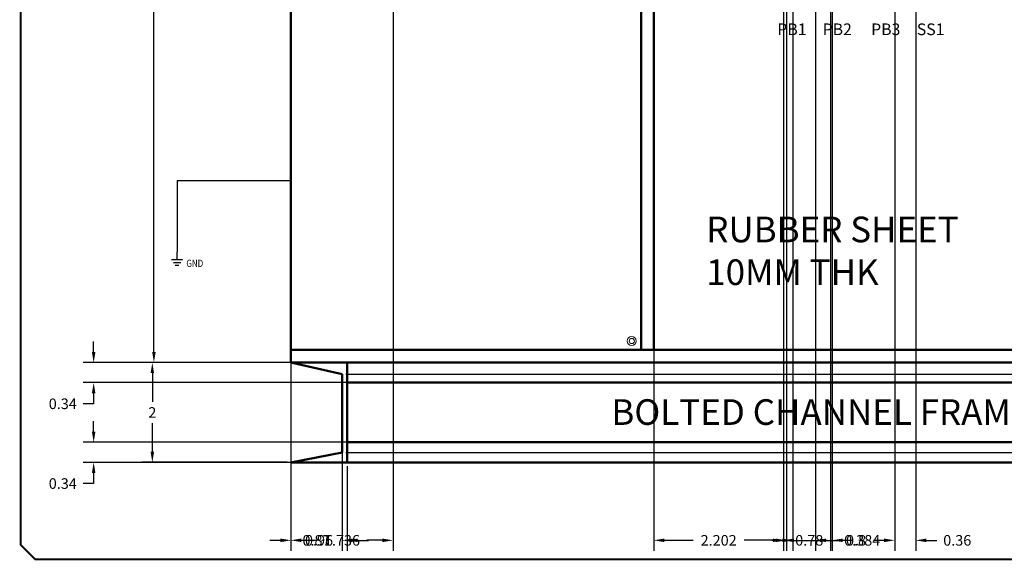
# Model space of a CAD drawing. Units: inches. Extents: x 0 to 33.5, y 0 to 22.4.
# Tile 1 of 6: x 0 to 16.8, y 0 to 9.2. Entities that reach past the tile are written whole.
import ezdxf
from ezdxf.enums import TextEntityAlignment as Align

# ---------------------------------------------------------------- set-up
doc = ezdxf.new("R2010")
doc.units = ezdxf.units.IN
doc.header["$MEASUREMENT"] = 0
for name, color, linetype, lineweight in [('E-ANNO-DIMS', 2, 'Continuous', 18), ('E-ANNO-TEXT', 7, 'Continuous', 18), ('E-ANNO-TTLB', 7, 'Continuous', 35), ('E-GRND-WIRE', 3, 'Continuous', 25), ('E-PANL-HDWR', 8, 'Continuous', 18), ('E-PANL-OUTL', 7, 'Continuous', 50), ('SYMS', 7, 'Continuous', 25)]:
    doc.layers.add(name, color=color, linetype=linetype, lineweight=lineweight)
doc.layers.add('TAGS', color=150, linetype='Continuous')
doc.layers.add('TITLE', color=7, linetype='Continuous')
doc.styles.add('ITALIC', font='ITALIC')
doc.styles.add('SIMPLEX', font='SIMPLEX')
doc.styles.add('WD', font='romans.shx')
doc.dimstyles.get("Standard").update_dxf_attribs({"dimtxt": 0.18, "dimasz": 0.18, "dimexe": 0.18, "dimexo": 0.0625, "dimgap": 0.09, "dimtad": 0, "dimtih": 1, "dimtoh": 1, "dimdec": 0, "dimzin": 0, "dimdsep": 46, "dimtxsty": 'Standard', "dimcen": 0.09, "dimadec": 0, "dimazin": 0, "dimtfac": 1, "dimtdec": 0, "dimtofl": 0, "dimtmove": 0, "dimatfit": 3, "dimfxl": 1, "dimtolj": 1, "dimtzin": 0, "dimarcsym": 0})

# ---------------------------------------------------------------- blocks, each defined once
blk = doc.blocks.new('NO_NUM_acade_title')
at = {"layer": 'TITLE', "const_width": 0.0312}
blk.add_lwpolyline([(30.594, 0.281), (30.594, 22.177), (30.344, 22.427), (0.281, 22.427), (0.031, 22.177), (0.031, 0.281), (0.281, 0.031), (30.344, 0.031)], close=True, dxfattribs=at)
at = {"layer": 'TITLE', "style": 'ITALIC'}
for tag, height, p in [('TITLE#1', 0.125, (32.156, 3.406)), ('TITLE#2', 0.125, (32.156, 3.204)), ('TITLE#3', 0.125, (32.156, 3.001)), ('TITLE#4', 0.125, (32.156, 2.799)), ('DWG#', 0.2, (32.156, 0.826))]:
    blk.add_attdef(tag, text='', height=height, dxfattribs=at).set_placement(p, align=Align.CENTER)
at = {"layer": 'TITLE', "style": 'SIMPLEX'}
blk.add_attdef('CAD#', (30.826, 1.958), '', height=0.0938, rotation=90, dxfattribs=at)
at = {"layer": 'TITLE'}
for tag, p, height, style in [('JOB#', (31.464, 1.644), 0.0938, 'SIMPLEX'), ('SCALE', (31.353, 1.344), 0.0938, 'SIMPLEX'), ('DATE', (32.408, 1.344), 0.0938, 'SIMPLEX'), ('SHTS', (32.532, 0.25), 0.2, 'ITALIC')]:
    blk.add_attdef(tag, p, '', height=height, dxfattribs=dict(at, style=style))
at = {"layer": 'TITLE', "style": 'ITALIC'}
blk.add_attdef('SH#', text='', height=0.2, dxfattribs=at).set_placement((31.881, 0.25), align=Align.RIGHT)
at = {"layer": 'TITLE', "flags": 9}
blk.add_attdef('WD_TB', (31.219, 0.031), '', height=0.125, dxfattribs=at)
blk = doc.blocks.new('VGND2')
for p, q in [((0, -0.125), (0, 0)), ((0.09375, -0.125), (-0.09375, -0.125)), ((-0.0625, -0.171875), (0.0625, -0.171875)), ((-0.03125, -0.21875), (0.03125, -0.21875))]:
    blk.add_line(p, q)
at = {"style": 'WD', "width": 0.8}
for tag, p in [('INST', (0.15625, 0.125)), ('LOC', (0.15625, -0.03125)), ('TAG1', (0.15625, -0.1875)), ('DESC1', (0.15625, -0.34375)), ('DESC2', (0.15625, -0.5))]:
    blk.add_attdef(tag, text='', height=0.125, dxfattribs=at).set_placement(p, align=Align.MIDDLE_LEFT)
at = {"style": 'WD', "flags": 1}
for tag in ['ASSYCODE', 'X2TERM01', 'CAT', 'MFG', 'FAMILY']:
    blk.add_attdef(tag, (0, 0), '', height=0.01, dxfattribs=at)
blk = doc.blocks.new('*D17')
at = {"layer": 'Defpoints', "color": 0, "transparency": 16777216}
for p in [(4.625, 18.375), (2.297, 3.375), (4.625, 3.375)]:
    blk.add_point(p, dxfattribs=at)
at = {"layer": 'E-ANNO-DIMS', "color": 0, "lineweight": -2, "transparency": 16777216}
for p, q in [((4.563, 18.375), (2.117, 18.375)), ((2.297, 18.195), (2.297, 11.055)), ((2.297, 3.555), (2.297, 10.695)), ((4.563, 3.375), (2.117, 3.375))]:
    blk.add_line(p, q, dxfattribs=at)
at = {"layer": 'E-ANNO-DIMS', "color": 0, "transparency": 16777216}
for points in [[(2.267, 18.195), (2.327, 18.195), (2.297, 18.375)], [(2.267, 3.555), (2.327, 3.555), (2.297, 3.375)]]:
    blk.add_solid(points, dxfattribs=at)
at = {"layer": 'E-ANNO-DIMS', "color": 0, "transparency": 16777216, "insert": (2.297, 10.875), "char_height": 0.18, "attachment_point": 5}
blk.add_mtext('\\A1;15', dxfattribs=at)
blk = doc.blocks.new('*D21')
at = {"layer": 'Defpoints', "color": 0, "transparency": 16777216}
for p in [(2.27, 3.375), (4.625, 3.375), (4.625, 1.68)]:
    blk.add_point(p, dxfattribs=at)
at = {"layer": 'E-ANNO-DIMS', "color": 0, "lineweight": -2, "transparency": 16777216}
for p, q in [((4.563, 3.375), (2.09, 3.375)), ((2.27, 3.195), (2.27, 2.707)), ((2.27, 1.86), (2.27, 2.347)), ((4.563, 1.68), (2.09, 1.68))]:
    blk.add_line(p, q, dxfattribs=at)
at = {"layer": 'E-ANNO-DIMS', "color": 0, "transparency": 16777216}
for points in [[(2.24, 3.195), (2.3, 3.195), (2.27, 3.375)], [(2.24, 1.86), (2.3, 1.86), (2.27, 1.68)]]:
    blk.add_solid(points, dxfattribs=at)
at = {"layer": 'E-ANNO-DIMS', "color": 0, "transparency": 16777216, "insert": (2.27, 2.527), "char_height": 0.18, "attachment_point": 5}
blk.add_mtext('\\A1;2', dxfattribs=at)
blk = doc.blocks.new('SCREW-PANEL')
for radius in [0.0768, 0.0442]:
    blk.add_circle((0.077, 0.077), radius)
blk = doc.blocks.new('*D27')
at = {"layer": 'Defpoints', "color": 0, "transparency": 16777216}
for p in [(13.540199, 20.522539), (13.156258, 18.375), (13.540199, 0.354641)]:
    blk.add_point(p, dxfattribs=at)
at = {"layer": 'E-ANNO-DIMS', "color": 0, "lineweight": -2, "transparency": 16777216}
for p, q in [((13.540199, 20.460039), (13.540199, 0.174641)), ((13.156258, 18.3125), (13.156258, 0.174641)), ((12.976258, 0.354641), (12.796258, 0.354641)), ((13.720199, 0.354641), (13.900199, 0.354641))]:
    blk.add_line(p, q, dxfattribs=at)
at = {"layer": 'E-ANNO-DIMS', "color": 0, "transparency": 16777216}
for points in [[(12.976258, 0.384641), (12.976258, 0.324641), (13.156258, 0.354641)], [(13.720199, 0.384641), (13.720199, 0.324641), (13.540199, 0.354641)]]:
    blk.add_solid(points, dxfattribs=at)
at = {"layer": 'E-ANNO-DIMS', "color": 0, "transparency": 16777216, "insert": (14.335199, 0.354641), "char_height": 0.18, "attachment_point": 5}
blk.add_mtext('\\A1;0.384', dxfattribs=at)
blk = doc.blocks.new('*D28')
at = {"layer": 'Defpoints', "color": 0, "transparency": 16777216}
for p in [(14.887335, 20.522539), (15.245612, 18.375), (15.245612, 0.354641)]:
    blk.add_point(p, dxfattribs=at)
at = {"layer": 'E-ANNO-DIMS', "color": 0, "lineweight": -2, "transparency": 16777216}
for p, q in [((14.887335, 20.460039), (14.887335, 0.174641)), ((15.245612, 18.3125), (15.245612, 0.174641)), ((14.707335, 0.354641), (14.527335, 0.354641)), ((15.425612, 0.354641), (15.605612, 0.354641))]:
    blk.add_line(p, q, dxfattribs=at)
at = {"layer": 'E-ANNO-DIMS', "color": 0, "transparency": 16777216}
for points in [[(14.707335, 0.384641), (14.707335, 0.324641), (14.887335, 0.354641)], [(15.425612, 0.384641), (15.425612, 0.324641), (15.245612, 0.354641)]]:
    blk.add_solid(points, dxfattribs=at)
at = {"layer": 'E-ANNO-DIMS', "color": 0, "transparency": 16777216, "insert": (15.950612, 0.354641), "char_height": 0.18, "attachment_point": 5}
blk.add_mtext('\\A1;0.36', dxfattribs=at)
blk = doc.blocks.new('*D31')
at = {"layer": 'Defpoints', "color": 0, "transparency": 16777216}
for p in [(14.887335, 20.522539), (27.49197, 20.522539), (23.941819, 1.679641)]:
    blk.add_point(p, dxfattribs=at)
at = {"layer": 'E-ANNO-DIMS', "color": 0, "lineweight": -2, "transparency": 16777216}
for p, q in [((14.949835, 20.522539), (27.67197, 20.522539)), ((27.49197, 20.342539), (27.49197, 11.28109)), ((27.49197, 1.859641), (27.49197, 10.92109)), ((24.004319, 1.679641), (27.67197, 1.679641))]:
    blk.add_line(p, q, dxfattribs=at)
at = {"layer": 'E-ANNO-DIMS', "color": 0, "transparency": 16777216}
for points in [[(27.46197, 20.342539), (27.52197, 20.342539), (27.49197, 20.522539)], [(27.46197, 1.859641), (27.52197, 1.859641), (27.49197, 1.679641)]]:
    blk.add_solid(points, dxfattribs=at)
at = {"layer": 'E-ANNO-DIMS', "color": 0, "transparency": 16777216, "insert": (27.49197, 11.10109), "char_height": 0.18, "attachment_point": 5}
blk.add_mtext('\\A1;18.843', dxfattribs=at)
blk = doc.blocks.new('*D33')
at = {"layer": 'Defpoints', "color": 0, "transparency": 16777216}
for p in [(23.061914, 3.375), (1.272879, 3.034671), (23.061914, 3.034671)]:
    blk.add_point(p, dxfattribs=at)
at = {"layer": 'E-ANNO-DIMS', "color": 0, "lineweight": -2, "transparency": 16777216}
for p, q in [((1.272879, 3.555), (1.272879, 3.735)), ((22.999414, 3.375), (1.092879, 3.375)), ((22.999414, 3.034671), (1.092879, 3.034671)), ((1.272879, 2.854671), (1.272879, 2.674671)), ((1.272879, 2.674671), (1.092879, 2.674671))]:
    blk.add_line(p, q, dxfattribs=at)
at = {"layer": 'E-ANNO-DIMS', "color": 0, "transparency": 16777216}
for points in [[(1.242879, 3.555), (1.302879, 3.555), (1.272879, 3.375)], [(1.242879, 2.854671), (1.302879, 2.854671), (1.272879, 3.034671)]]:
    blk.add_solid(points, dxfattribs=at)
at = {"layer": 'E-ANNO-DIMS', "color": 0, "transparency": 16777216, "insert": (0.747879, 2.674671), "char_height": 0.18, "attachment_point": 5}
blk.add_mtext('\\A1;0.34', dxfattribs=at)
blk = doc.blocks.new('*D34')
at = {"layer": 'Defpoints', "color": 0, "transparency": 16777216}
for p in [(23.061914, 2.019969), (1.272879, 1.679641), (23.061914, 1.679641)]:
    blk.add_point(p, dxfattribs=at)
at = {"layer": 'E-ANNO-DIMS', "color": 0, "lineweight": -2, "transparency": 16777216}
for p, q in [((1.272879, 2.199969), (1.272879, 2.379969)), ((22.999414, 2.019969), (1.092879, 2.019969)), ((22.999414, 1.679641), (1.092879, 1.679641)), ((1.272879, 1.499641), (1.272879, 1.319641)), ((1.272879, 1.319641), (1.092879, 1.319641))]:
    blk.add_line(p, q, dxfattribs=at)
at = {"layer": 'E-ANNO-DIMS', "color": 0, "transparency": 16777216}
for points in [[(1.242879, 2.199969), (1.302879, 2.199969), (1.272879, 2.019969)], [(1.242879, 1.499641), (1.302879, 1.499641), (1.272879, 1.679641)]]:
    blk.add_solid(points, dxfattribs=at)
at = {"layer": 'E-ANNO-DIMS', "color": 0, "transparency": 16777216, "insert": (0.747879, 1.319641), "char_height": 0.18, "attachment_point": 5}
blk.add_mtext('\\A1;0.34', dxfattribs=at)
blk = doc.blocks.new('*D35')
at = {"layer": 'Defpoints', "color": 0, "transparency": 16777216}
for p in [(4.625144, 1.679641), (5.58188, 1.679641), (5.58188, 0.354641)]:
    blk.add_point(p, dxfattribs=at)
at = {"layer": 'E-ANNO-DIMS', "color": 0, "lineweight": -2, "transparency": 16777216}
for p, q in [((4.625144, 1.617141), (4.625144, 0.174641)), ((5.58188, 1.617141), (5.58188, 0.174641)), ((4.445144, 0.354641), (4.265144, 0.354641)), ((5.76188, 0.354641), (5.94188, 0.354641))]:
    blk.add_line(p, q, dxfattribs=at)
at = {"layer": 'E-ANNO-DIMS', "color": 0, "transparency": 16777216}
for points in [[(4.445144, 0.384641), (4.445144, 0.324641), (4.625144, 0.354641)], [(5.76188, 0.384641), (5.76188, 0.324641), (5.58188, 0.354641)]]:
    blk.add_solid(points, dxfattribs=at)
at = {"layer": 'E-ANNO-DIMS', "color": 0, "transparency": 16777216, "insert": (5.103512, 0.354641), "char_height": 0.18, "attachment_point": 5}
blk.add_mtext('\\A1;0.96', dxfattribs=at)
blk = doc.blocks.new('*D36')
at = {"layer": 'Defpoints', "color": 0, "transparency": 16777216}
for p in [(4.625144, 3.375), (5.49433, 3.177405), (5.49433, 0.354641)]:
    blk.add_point(p, dxfattribs=at)
at = {"layer": 'E-ANNO-DIMS', "color": 0, "lineweight": -2, "transparency": 16777216}
for p, q in [((4.625144, 3.3125), (4.625144, 0.174641)), ((5.49433, 3.114905), (5.49433, 0.174641)), ((4.445144, 0.354641), (4.265144, 0.354641)), ((5.67433, 0.354641), (5.85433, 0.354641))]:
    blk.add_line(p, q, dxfattribs=at)
at = {"layer": 'E-ANNO-DIMS', "color": 0, "transparency": 16777216}
for points in [[(4.445144, 0.384641), (4.445144, 0.324641), (4.625144, 0.354641)], [(5.67433, 0.384641), (5.67433, 0.324641), (5.49433, 0.354641)]]:
    blk.add_solid(points, dxfattribs=at)
at = {"layer": 'E-ANNO-DIMS', "color": 0, "transparency": 16777216, "insert": (5.059737, 0.354641), "char_height": 0.18, "attachment_point": 5}
blk.add_mtext('\\A1;0.87', dxfattribs=at)
blk = doc.blocks.new('*D37')
at = {"layer": 'Defpoints', "color": 0, "transparency": 16777216}
for p in [(5.494, 3.177), (5.494, 1.847), (27.492, 1.847)]:
    blk.add_point(p, dxfattribs=at)
at = {"layer": 'E-ANNO-DIMS', "color": 0, "lineweight": -2, "transparency": 16777216}
for p, q in [((5.557, 3.177), (27.672, 3.177)), ((27.492, 2.997), (27.492, 2.692)), ((27.492, 2.027), (27.492, 2.332)), ((5.557, 1.847), (27.672, 1.847))]:
    blk.add_line(p, q, dxfattribs=at)
at = {"layer": 'E-ANNO-DIMS', "color": 0, "transparency": 16777216}
for points in [[(27.462, 2.997), (27.522, 2.997), (27.492, 3.177)], [(27.462, 2.027), (27.522, 2.027), (27.492, 1.847)]]:
    blk.add_solid(points, dxfattribs=at)
at = {"layer": 'E-ANNO-DIMS', "color": 0, "transparency": 16777216, "insert": (27.492, 2.512), "char_height": 0.18, "attachment_point": 5}
blk.add_mtext('\\A1;1.33', dxfattribs=at)
blk = doc.blocks.new('*D46')
at = {"layer": 'Defpoints', "color": 0, "transparency": 16777216}
for p in [(4.625, 18.375), (6.361, 10.63), (6.361, 0.355)]:
    blk.add_point(p, dxfattribs=at)
at = {"layer": 'E-ANNO-DIMS', "color": 0, "lineweight": -2, "transparency": 16777216}
for p, q in [((4.625, 18.312), (4.625, 0.175)), ((6.361, 10.568), (6.361, 0.175)), ((4.805, 0.355), (5.073, 0.355)), ((6.181, 0.355), (5.913, 0.355))]:
    blk.add_line(p, q, dxfattribs=at)
at = {"layer": 'E-ANNO-DIMS', "color": 0, "transparency": 16777216}
for points in [[(4.805, 0.385), (4.805, 0.325), (4.625, 0.355)], [(6.181, 0.385), (6.181, 0.325), (6.361, 0.355)]]:
    blk.add_solid(points, dxfattribs=at)
at = {"layer": 'E-ANNO-DIMS', "color": 0, "transparency": 16777216, "insert": (5.493, 0.355), "char_height": 0.18, "attachment_point": 5}
blk.add_mtext('\\A1;1.736', dxfattribs=at)
blk = doc.blocks.new('*D58')
at = {"layer": 'Defpoints', "color": 0, "transparency": 16777216}
for p in [(10.794, 18.375), (12.996, 10.465), (12.996, 0.355)]:
    blk.add_point(p, dxfattribs=at)
at = {"layer": 'E-ANNO-DIMS', "color": 0, "lineweight": -2, "transparency": 16777216}
for p, q in [((10.794, 18.312), (10.794, 0.175)), ((12.996, 10.403), (12.996, 0.175)), ((10.974, 0.355), (11.46, 0.355)), ((12.816, 0.355), (12.33, 0.355))]:
    blk.add_line(p, q, dxfattribs=at)
at = {"layer": 'E-ANNO-DIMS', "color": 0, "transparency": 16777216}
for points in [[(10.974, 0.385), (10.974, 0.325), (10.794, 0.355)], [(12.816, 0.385), (12.816, 0.325), (12.996, 0.355)]]:
    blk.add_solid(points, dxfattribs=at)
at = {"layer": 'E-ANNO-DIMS', "color": 0, "transparency": 16777216, "insert": (11.895, 0.355), "char_height": 0.18, "attachment_point": 5}
blk.add_mtext('\\A1;2.202', dxfattribs=at)
blk = doc.blocks.new('*D65')
at = {"layer": 'Defpoints', "color": 0, "transparency": 16777216}
for p in [(12.995825, 10.465374), (13.795825, 10.465374), (13.795825, 0.354641)]:
    blk.add_point(p, dxfattribs=at)
at = {"layer": 'E-ANNO-DIMS', "color": 0, "lineweight": -2, "transparency": 16777216}
for p, q in [((12.995825, 10.402874), (12.995825, 0.174641)), ((13.795825, 10.402874), (13.795825, 0.174641)), ((13.175825, 0.354641), (13.615825, 0.354641)), ((13.795825, 0.354641), (13.975825, 0.354641))]:
    blk.add_line(p, q, dxfattribs=at)
at = {"layer": 'E-ANNO-DIMS', "color": 0, "transparency": 16777216}
for points in [[(13.175825, 0.384641), (13.175825, 0.324641), (12.995825, 0.354641)], [(13.615825, 0.384641), (13.615825, 0.324641), (13.795825, 0.354641)]]:
    blk.add_solid(points, dxfattribs=at)
at = {"layer": 'E-ANNO-DIMS', "color": 0, "transparency": 16777216, "insert": (14.230825, 0.354641), "char_height": 0.18, "attachment_point": 5}
blk.add_mtext('\\A1;0.8', dxfattribs=at)
blk = doc.blocks.new('*D66')
at = {"layer": 'Defpoints', "color": 0, "transparency": 16777216}
for p in [(13.047, 9.51), (13.823, 9.51), (13.823, 0.355)]:
    blk.add_point(p, dxfattribs=at)
at = {"layer": 'E-ANNO-DIMS', "color": 0, "lineweight": -2, "transparency": 16777216}
for p, q in [((13.047, 9.447), (13.047, 0.175)), ((13.823, 9.447), (13.823, 0.175)), ((12.867, 0.355), (12.687, 0.355)), ((14.003, 0.355), (14.183, 0.355))]:
    blk.add_line(p, q, dxfattribs=at)
at = {"layer": 'E-ANNO-DIMS', "color": 0, "transparency": 16777216}
for points in [[(12.867, 0.385), (12.867, 0.325), (13.047, 0.355)], [(14.003, 0.385), (14.003, 0.325), (13.823, 0.355)]]:
    blk.add_solid(points, dxfattribs=at)
at = {"layer": 'E-ANNO-DIMS', "color": 0, "transparency": 16777216, "insert": (13.435, 0.355), "char_height": 0.18, "attachment_point": 5}
blk.add_mtext('\\A1;0.78', dxfattribs=at)

msp = doc.modelspace()

# ---------------------------------------------------------------- linework, layer by layer
at = {"layer": 'E-GRND-WIRE'}
for p, q in [((4.6251, 6.4624), (2.6916, 6.4624)), ((2.6916, 6.4624), (2.6916, 5.2476)), ((4.6251, 6.4624), (4.6251, 6.4624))]:
    msp.add_line(p, q, dxfattribs=at)
at = {"layer": 'E-PANL-OUTL'}
for p, q in [((4.6251, 3.375), (4.6251, 18.375)), ((10.5789, 3.5899), (10.5789, 18.375)), ((10.7938, 3.5899), (10.7938, 18.375)), ((23.7937, 3.5899), (4.6251, 3.5899)), ((23.7937, 3.375), (4.6251, 3.375)), ((4.6251, 3.375), (5.4943, 3.1774)), ((5.5819, 1.6796), (5.5819, 3.375)), ((5.4943, 3.1774), (5.4943, 1.8466)), ((23.0619, 3.0347), (5.5819, 3.0347)), ((23.0619, 2.02), (5.5819, 2.02)), ((5.4943, 1.8466), (4.6251, 1.6796)), ((5.5819, 1.6796), (4.6251, 1.6796)), ((23.0619, 1.6796), (5.5819, 1.6796))]:
    msp.add_line(p, q, dxfattribs=at)

# ---------------------------------------------------------------- block references
at = {"layer": 'E-ANNO-TTLB'}
msp.add_blockref('NO_NUM_acade_title', (0, 0), dxfattribs=at)
at = {"layer": 'E-PANL-HDWR'}
msp.add_blockref('SCREW-PANEL', (10.341, 3.6637), dxfattribs=at)
at = {"layer": 'SYMS'}
ref = msp.add_blockref('VGND2', (2.6916, 5.2476), dxfattribs=at)
ref.add_attrib('TAG1', 'GND', dxfattribs={"layer": 'TAGS', "height": 0.125, "style": 'WD', "width": 0.8}).set_placement((2.8479, 5.0601), align=Align.MIDDLE_LEFT)

# ---------------------------------------------------------------- texts
at = {"layer": 'E-ANNO-TEXT'}
for s, height, p in [('PB1', 0.19791, (12.8913, 8.9374)), ('PB2', 0.19791, (13.6612, 8.9374)), ('PB3', 0.19791, (14.4861, 8.9374)), ('SS1', 0.19791, (15.2624, 8.9374)), ('RUBBER SHEET', 0.435566, (11.6843, 5.418)), ('10MM THK', 0.43557, (11.6843, 4.6921)), ('BOLTED CHANNEL FRAME', 0.435566, (10.0718, 2.316))]:
    msp.add_text(s, height=height, dxfattribs=at).set_placement(p)

# ---------------------------------------------------------------- dimensions: what is measured, and where the dimension line sits
at = {"layer": 'E-ANNO-DIMS'}
for base, p1, p2, override, picture, middle in [((13.5402, 0.3546), (13.1563, 18.375), (13.5402, 20.5225), {"dimdec": 3, "dimlfac": 1, "dimrnd": 0, "dimzin": 0, "dimdsep": 46, "dimlunit": 2}, '*D27', (14.3352, 0.3546)), ((15.2456, 0.3546), (14.8873, 20.5225), (15.2456, 18.375), {"dimdec": 2, "dimlfac": 1, "dimrnd": 0, "dimzin": 0, "dimdsep": 46, "dimlunit": 2}, '*D28', (15.9506, 0.3546)), ((6.3613, 0.3546), (4.6251, 18.375), (6.3613, 10.6304), {"dimdec": 3, "dimlfac": 1, "dimrnd": 0, "dimzin": 0, "dimdsep": 46, "dimlunit": 2}, '*D46', (5.4932, 0.3546)), ((12.9958, 0.3546), (10.7938, 18.375), (12.9958, 10.4654), {"dimdec": 3, "dimlfac": 1, "dimrnd": 0, "dimzin": 0, "dimdsep": 46, "dimlunit": 2}, '*D58', (11.8948, 0.3546)), ((13.7958, 0.3546), (12.9958, 10.4654), (13.7958, 10.4654), {"dimdec": 1, "dimlfac": 1, "dimrnd": 0, "dimzin": 0, "dimdsep": 46, "dimlunit": 2}, '*D65', (14.2308, 0.3546)), ((13.8235, 0.3546), (13.0472, 9.5097), (13.8235, 9.5097), {"dimdec": 2, "dimlfac": 1, "dimrnd": 0, "dimzin": 0, "dimdsep": 46, "dimlunit": 2}, '*D66', (13.4354, 0.3546)), ((5.4943, 0.3546), (4.6251, 3.375), (5.4943, 3.1774), {"dimdec": 2, "dimlfac": 1, "dimrnd": 0, "dimzin": 0, "dimdsep": 46, "dimlunit": 2}, '*D36', (5.0597, 0.3546)), ((5.5819, 0.3546), (4.6251, 1.6796), (5.5819, 1.6796), {"dimdec": 2, "dimlfac": 1, "dimrnd": 0, "dimzin": 0, "dimdsep": 46, "dimlunit": 2}, '*D35', (5.1035, 0.3546))]:
    dim = msp.add_linear_dim(base=base, p1=p1, p2=p2, dimstyle='Standard', override=override, dxfattribs=at)
    dim.commit()
    dim.dimension.update_dxf_attribs({"geometry": picture, "text_midpoint": middle})
for base, p1, p2, override, picture, middle in [((27.492, 20.5225), (23.9418, 1.6796), (14.8873, 20.5225), {"dimdec": 3, "dimlfac": 1, "dimrnd": 0, "dimzin": 0, "dimdsep": 46, "dimlunit": 2}, '*D31', (27.492, 11.1011)), ((2.2967, 3.375), (4.6251, 18.375), (4.6251, 3.375), {"dimclrd": 0, "dimclre": 0, "dimclrt": 0}, '*D17', (2.2967, 10.875)), ((1.2729, 3.0347), (23.0619, 3.375), (23.0619, 3.0347), {"dimdec": 2, "dimlfac": 1, "dimrnd": 0, "dimzin": 0, "dimdsep": 46, "dimlunit": 2}, '*D33', (0.7479, 2.6747)), ((2.2703, 3.375), (4.6251, 1.6796), (4.6251, 3.375), {"dimclrd": 0, "dimclre": 0, "dimclrt": 0}, '*D21', (2.2703, 2.5273)), ((27.492, 1.8466), (5.4943, 3.1774), (5.4943, 1.8466), {"dimdec": 2, "dimlfac": 1, "dimrnd": 0, "dimzin": 0, "dimdsep": 46, "dimlunit": 2}, '*D37', (27.492, 2.512)), ((1.2729, 1.6796), (23.0619, 2.02), (23.0619, 1.6796), {"dimdec": 2, "dimlfac": 1, "dimrnd": 0, "dimzin": 0, "dimdsep": 46, "dimlunit": 2}, '*D34', (0.7479, 1.3196))]:
    dim = msp.add_linear_dim(base=base, p1=p1, p2=p2, angle=90, dimstyle='Standard', override=override, dxfattribs=at)
    dim.commit()
    dim.dimension.update_dxf_attribs({"geometry": picture, "text_midpoint": middle})

doc.saveas('drawing.dxf')
